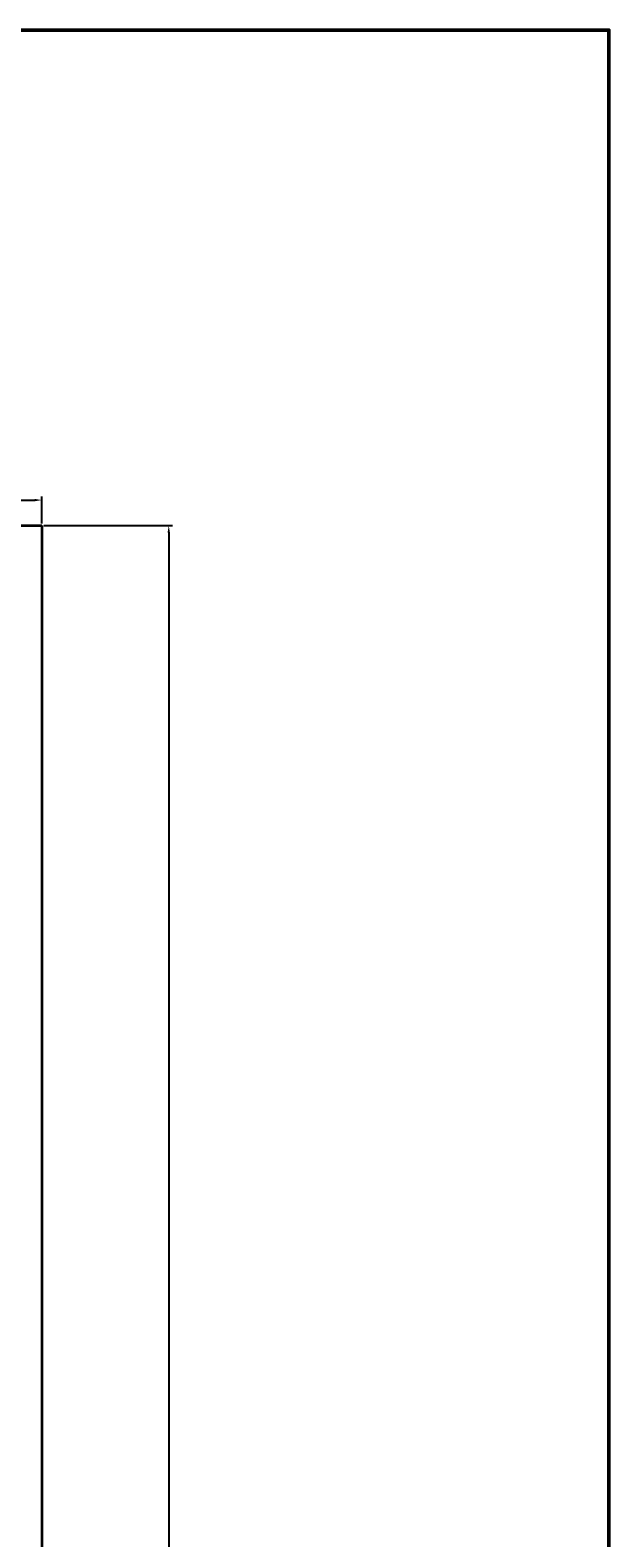
# Model space of a CAD drawing. Units: millimetres. Extents: x 2134 to 3363, y 1052 to 3233.
# Tile 11 of 11: x 3165 to 3363, y 2718 to 3233. Entities that reach past the tile are written whole.
import ezdxf

# ---------------------------------------------------------------- set-up
doc = ezdxf.new("R2010")
doc.units = ezdxf.units.MM
for name, color, linetype, lineweight in [('A-ANNO-DIMS', 2, 'Continuous', 18), ('A-ANNO-TTLB', 7, 'Continuous', 50), ('C-PROP', 6, 'Continuous', 35)]:
    doc.layers.add(name, color=color, linetype=linetype, lineweight=lineweight)
doc.styles.get("Standard").update_dxf_attribs({"font": 'arial.ttf'})
doc.dimstyles.new('ISO-25', dxfattribs={"dimtxt": 2.5, "dimasz": 2.5, "dimexe": 1.25, "dimexo": 0.625, "dimtad": 1, "dimtxsty": 'Standard', "dimcen": 2.5, "dimadec": 0, "dimazin": 0, "dimtfac": 1, "dimtmove": 0, "dimatfit": 3, "dimfxl": 1, "dimarcsym": 0})

# ---------------------------------------------------------------- blocks, each defined once
blk = doc.blocks.new('*D9')
at = {"layer": 'A-ANNO-DIMS', "color": 0, "lineweight": -2, "transparency": 16777216}
for p, q in [((3169.46, 3063.82), (3213.48, 3063.82)), ((3212.23, 3061.32), (3212.23, 1770.32)), ((3169.46, 1767.82), (3213.48, 1767.82))]:
    blk.add_line(p, q, dxfattribs=at)
at = {"layer": 'A-ANNO-DIMS', "color": 0, "transparency": 16777216}
for points in [[(3211.81, 3061.32), (3212.65, 3061.32), (3212.23, 3063.82)], [(3211.81, 1770.32), (3212.65, 1770.32), (3212.23, 1767.82)]]:
    blk.add_solid(points, dxfattribs=at)
at = {"layer": 'Defpoints', "color": 0, "transparency": 16777216}
for p in [(3168.84, 3063.82), (3168.84, 1767.82), (3212.23, 1767.82)]:
    blk.add_point(p, dxfattribs=at)
at = {"layer": 'A-ANNO-DIMS', "color": 0, "transparency": 16777216, "insert": (3210.33, 2415.82), "char_height": 2.5, "attachment_point": 5, "rotation": 90}
blk.add_mtext('1296', dxfattribs=at)
blk = doc.blocks.new('*D16')
at = {"layer": 'A-ANNO-DIMS', "color": 0, "lineweight": -2, "transparency": 16777216}
for p, q in [((2491.84, 3064.45), (2491.84, 3073.74)), ((3168.84, 3064.45), (3168.84, 3073.74)), ((2494.34, 3072.49), (3166.34, 3072.49))]:
    blk.add_line(p, q, dxfattribs=at)
at = {"layer": 'A-ANNO-DIMS', "color": 0, "transparency": 16777216}
for points in [[(2494.34, 3072.9), (2494.34, 3072.07), (2491.84, 3072.49)], [(3166.34, 3072.9), (3166.34, 3072.07), (3168.84, 3072.49)]]:
    blk.add_solid(points, dxfattribs=at)
at = {"layer": 'Defpoints', "color": 0, "transparency": 16777216}
for p in [(3168.84, 3072.49), (2491.84, 3063.82), (3168.84, 3063.82)]:
    blk.add_point(p, dxfattribs=at)
at = {"layer": 'A-ANNO-DIMS', "color": 0, "transparency": 16777216, "insert": (2830.34, 3074.39), "char_height": 2.5, "attachment_point": 5}
blk.add_mtext('677', dxfattribs=at)

msp = doc.modelspace()

# ---------------------------------------------------------------- linework, layer by layer
at = {"layer": 'A-ANNO-TTLB', "ltscale": 0.5}
msp.add_lwpolyline([(2134.34, 3233.23), (3362.77, 3233.23), (3362.77, 1152.237), (2134.34, 1152.237)], close=True, dxfattribs=at)
at = {"layer": 'C-PROP'}
for p, q in [((2491.839, 3063.82), (3168.839, 3063.82)), ((3168.839, 3063.82), (3168.839, 1767.82))]:
    msp.add_line(p, q, dxfattribs=at)

# ---------------------------------------------------------------- dimensions: what is measured, and where the dimension line sits
at = {"layer": 'A-ANNO-DIMS'}
dim = msp.add_linear_dim(base=(3168.839, 3072.486), p1=(2491.839, 3063.82), p2=(3168.839, 3063.82), dimstyle='ISO-25', override={"dimclrd": 0, "dimclre": 0, "dimclrt": 0}, dxfattribs=at)
dim.commit()
dim.dimension.update_dxf_attribs({"geometry": '*D16', "text_midpoint": (2830.339, 3074.387)})
dim = msp.add_linear_dim(base=(3212.229, 1767.82), p1=(3168.839, 3063.82), p2=(3168.839, 1767.82), angle=90, dimstyle='ISO-25', override={"dimclrd": 0, "dimclre": 0, "dimclrt": 0}, dxfattribs=at)
dim.commit()
dim.dimension.update_dxf_attribs({"geometry": '*D9', "text_midpoint": (3210.327, 2415.82)})

doc.saveas('drawing.dxf')
